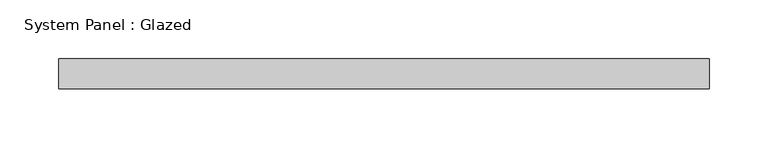
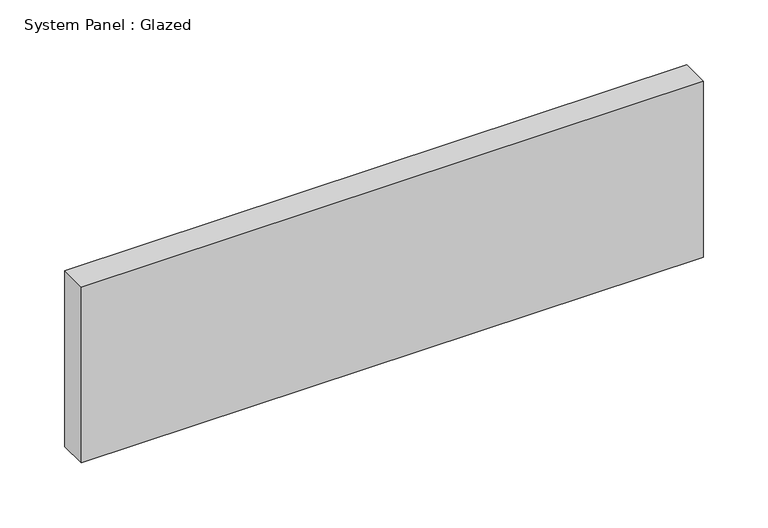
"""IFC4 building model written with IfcOpenShell, lengths in millimetres: plate geometry, System Panel : Glazed."""

from ifc_helpers import new_model, si_unit, origin, origin_with_axes, place, context, project, spatial, polyline, outline, extrude, source, transform, mapped, element, save


def system_panel_glazed_b3845325(model_context):
    return source(origin(), model_context, "Body", "SweptSolid", [
        extrude(outline(polyline([(276.2250002, 19.05), (-276.2250002, 19.05), (-276.2250002, 44.45), (276.2250002, 44.45), (276.2250002, 19.05)])), origin_with_axes(), (0.0, 0.0, 1.0), 165.1),
    ])


if __name__ == "__main__":
    model = new_model("IFC4")
    model_context = context("Model", 3, world=origin())
    ifc_project = project(units=[si_unit("LENGTHUNIT", "METRE", prefix="MILLI")], contexts=[model_context])
    site = spatial("IfcSite", under=ifc_project)
    building = spatial("IfcBuilding", under=site)
    placement = place(None, origin())
    system_panel_glazed_shape = system_panel_glazed_b3845325(model_context)
    element("IfcPlate", 1, ObjectType="System Panel : Glazed", at=placement, inside=building, context=model_context, shape_type="MappedRepresentation", body=[
        mapped(system_panel_glazed_shape, transform((0.0, 0.0, 0.0), x_axis=(1.0, 0.0, 0.0), y_axis=(0.0, 1.0, 0.0), z_axis=(0.0, 0.0, 1.0))),
    ])
    save(model, "model.ifc")

# Revit data of these elements
# Type "System Panel : Glazed"
#   Construction Type Id = "GSP4R"
#   Analytic Construction = "1/8 in Pilkington single glazing"
#   Visual Light Transmittance = 0.9
#   Solar Heat Gain Coefficient = 0.86
#   Heat Transfer Coefficient (U) = 1.18115 BTU/(h·ft²·°F)
#   Define Thermal Properties by = 1
# Element 1 (IfcPlate, "System Panel : Glazed")
#   Materials on its faces: "Glass"
# Materials
#   "Glass": class "Glass", colour RGB 0 128 192, transparency 0.75, Description = "Soda Lime Glass", Cost = 0
